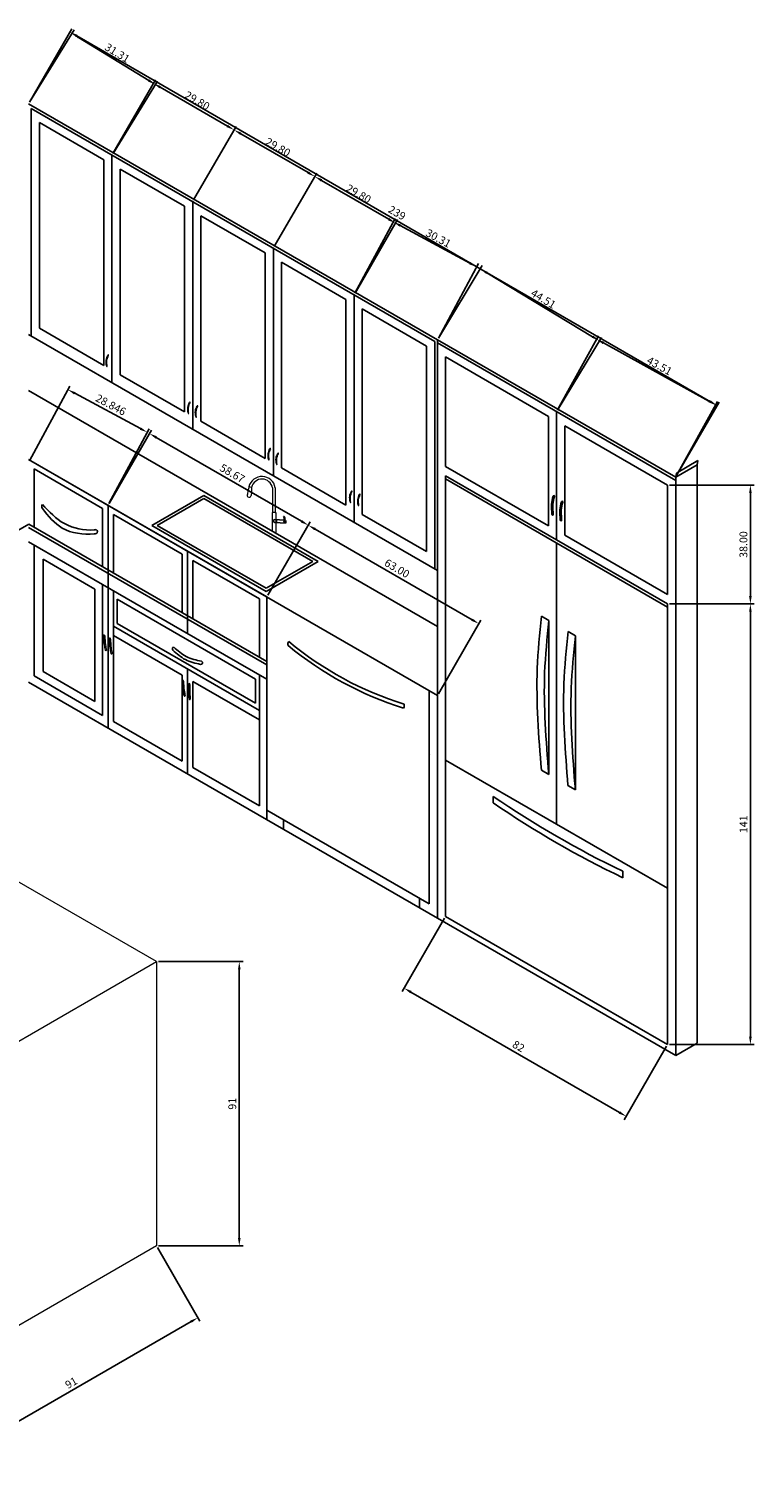
# Model space of a CAD drawing. Units: centimetres. Extents: x 21667 to 22807, y 15845 to 16565.
# Tile 4 of 4: x 22575 to 22807, y 16106 to 16565. Entities that reach past the tile are written whole.
import ezdxf

# ---------------------------------------------------------------- set-up
doc = ezdxf.new("R2010")
doc.units = ezdxf.units.CM
for name, color, linetype, lineweight in [('A-ANNO-DIMS', 2, 'Continuous', 18), ('A-ANNO-NPLT', 8, 'Continuous', 13), ('A-FLOR-FIXT', 4, 'Continuous', 18), ('A-FURN', 8, 'Continuous', 18), ('A-FURN-CASE', 7, 'Continuous', 25), ('A-FURN-HDWR', 8, 'Continuous', 13)]:
    doc.layers.add(name, color=color, linetype=linetype, lineweight=lineweight)
doc.styles.get("Standard").update_dxf_attribs({"font": 'arial.ttf'})
doc.dimstyles.new('ISO-25', dxfattribs={"dimtxt": 2.5, "dimasz": 2.5, "dimexe": 1.25, "dimexo": 0.625, "dimtad": 1, "dimtxsty": 'Standard', "dimcen": 2.5, "dimadec": 0, "dimazin": 0, "dimtfac": 1, "dimtmove": 0, "dimatfit": 3, "dimfxl": 1, "dimarcsym": 0})

# ---------------------------------------------------------------- blocks, each defined once
blk = doc.blocks.new('tabl e3')
for p, q in [((22512.57, 16212.95), (22433.76, 16167.45)), ((22643.34, 16137.45), (22512.57, 16212.95)), ((22433.76, 16167.45), (22564.53, 16091.95)), ((22433.76, 16167.45), (22433.76, 16076.45)), ((22459.07, 16152.84), (22459.07, 16091.06)), ((22564.53, 16091.95), (22643.34, 16137.45)), ((22643.34, 16137.45), (22643.34, 16046.45)), ((22493.36, 16133.04), (22493.36, 16076.26)), ((22495.09, 16132.04), (22495.09, 16075.26)), ((22528.51, 16112.74), (22528.51, 16055.97)), ((22530.25, 16111.74), (22530.25, 16054.97)), ((22459.07, 16096.06), (22564.53, 16035.17)), ((22433.76, 16076.45), (22459.07, 16091.06)), ((22459.07, 16091.06), (22564.53, 16030.17)), ((22564.53, 16000.95), (22564.53, 16091.95)), ((22433.76, 16076.45), (22564.53, 16000.95)), ((22643.34, 16046.45), (22564.53, 16000.95))]:
    blk.add_line(p, q)
for p in [(22494.23, 16132.54), (22529.38, 16112.24)]:
    blk.add_point(p)
blk = doc.blocks.new('PULL-KNOB-A')
for centre, radius, start, end in [((0.27, 0.14), 0.142, 166.0993, 319.2848), ((0.68, 3.52), 0.139, 326.4959, 158.8882)]:
    blk.add_arc(centre, radius, start, end)
for points in [[(0.14, 0.18), (0.04, 0.79), (-0.14, 1.97), (0.33, 3.06), (0.55, 3.57)], [(0.38, 0.05), (0.29, 0.67), (0.11, 1.84), (0.58, 2.93), (0.8, 3.44)]]:
    blk.add_open_spline(points, degree=3, knots=[0, 0, 0, 0, 1.835259, 3.479337, 3.479337, 3.479337, 3.479337])
blk = doc.blocks.new('PULL-KNOB-C')
for centre, radius, start, end in [((0.27, 4.86), 0.21, 340.7069, 183.1566), ((0.41, 0.22), 0.218, 191.5838, 332.2797)]:
    blk.add_arc(centre, radius, start, end)
for points in [[(0.06, 4.85), (0.01, 3.87), (-0.06, 2.31), (0.13, 0.76), (0.2, 0.17)], [(0.46, 4.79), (0.42, 3.82), (0.35, 2.25), (0.54, 0.7), (0.61, 0.12)]]:
    blk.add_open_spline(points, degree=3, knots=[0, 0, 0, 0, 2.913566, 4.680035, 4.680035, 4.680035, 4.680035])
blk = doc.blocks.new('FAUCET')
for p, q in [((1.4, 14.57), (0.59, 14.75)), ((8.15, 14.4), (8.15, 6.62)), ((8.99, 14.47), (8.99, 6.62)), ((8.15, 6.62), (8.01, 6.3)), ((8.01, 6.3), (8.01, 0.66)), ((8.15, 6.62), (8.99, 6.62)), ((8.99, 6.62), (9.15, 6.35)), ((9.15, 6.35), (9.15, 0))]:
    blk.add_line(p, q)
for radius, start in [(4.28, 8.9589), (3.44, 9.9927)]:
    blk.add_arc((4.76, 13.81), radius, start, 167.251)
for points, knots in [([(0.59, 14.75), (0.5, 14.32), (0.32, 13.44), (0.11, 12.57), (0, 12.12)], [0, 0, 0, 0, 1.316127, 2.691834, 2.691834, 2.691834, 2.691834]), ([(1.4, 14.57), (1.41, 14.09), (1.41, 13.24), (1.35, 12.4), (1.32, 12.02)], [0, 0, 0, 0, 1.416831, 2.547877, 2.547877, 2.547877, 2.547877]), ([(0, 12.12), (0.01, 11.98), (0.03, 11.46), (1.13, 11.35), (1.28, 11.86), (1.32, 12.02)], [0, 0, 0, 0, 0.416688, 1.456431, 1.924702, 1.924702, 1.924702, 1.924702])]:
    blk.add_open_spline(points, degree=3, knots=knots)
blk = doc.blocks.new('*D27')
at = {"layer": 'A-ANNO-DIMS', "color": 0, "lineweight": -2, "transparency": 16777216}
for p, q in [((22575.26, 16541.62), (22588.83, 16565.11)), ((22590.37, 16562.77), (22793.02, 16445.77)), ((22782.24, 16422.12), (22795.81, 16445.61))]:
    blk.add_line(p, q, dxfattribs=at)
at = {"layer": 'A-ANNO-DIMS', "color": 0, "transparency": 16777216}
for points in [[(22590.58, 16563.14), (22590.16, 16562.41), (22588.2, 16564.02)], [(22793.23, 16446.14), (22792.81, 16445.41), (22795.18, 16444.52)]]:
    blk.add_solid(points, dxfattribs=at)
at = {"layer": 'Defpoints', "color": 0, "transparency": 16777216}
for p in [(22574.95, 16541.07), (22795.18, 16444.52), (22781.93, 16421.57)]:
    blk.add_point(p, dxfattribs=at)
at = {"layer": 'A-ANNO-DIMS', "color": 0, "transparency": 16777216, "insert": (22692.64, 16505.92), "char_height": 2.5, "attachment_point": 5, "rotation": 330}
blk.add_mtext('239', dxfattribs=at)
blk = doc.blocks.new('*D32')
at = {"layer": 'A-ANNO-DIMS', "color": 0, "lineweight": -2, "transparency": 16777216}
for p, q in [((22708.01, 16280.53), (22694.44, 16257.04)), ((22763.92, 16218.38), (22697.23, 16256.88)), ((22779.02, 16239.53), (22765.46, 16216.04))]:
    blk.add_line(p, q, dxfattribs=at)
at = {"layer": 'A-ANNO-DIMS', "color": 0, "transparency": 16777216}
for points in [[(22697.44, 16257.24), (22697.03, 16256.51), (22695.07, 16258.13)], [(22764.13, 16218.74), (22763.71, 16218.01), (22766.08, 16217.13)]]:
    blk.add_solid(points, dxfattribs=at)
at = {"layer": 'Defpoints', "color": 0, "transparency": 16777216}
for p in [(22708.32, 16281.07), (22695.07, 16258.13), (22779.33, 16240.07)]:
    blk.add_point(p, dxfattribs=at)
at = {"layer": 'A-ANNO-DIMS', "color": 0, "transparency": 16777216, "insert": (22731.53, 16239.27), "char_height": 2.5, "attachment_point": 5, "rotation": 330}
blk.add_mtext('82', dxfattribs=at)
blk = doc.blocks.new('*D33')
at = {"layer": 'A-ANNO-DIMS', "color": 0, "lineweight": -2, "transparency": 16777216}
for p, q in [((22779.96, 16381.07), (22807.08, 16381.07)), ((22805.83, 16378.57), (22805.83, 16242.57)), ((22779.96, 16240.07), (22807.08, 16240.07))]:
    blk.add_line(p, q, dxfattribs=at)
at = {"layer": 'A-ANNO-DIMS', "color": 0, "transparency": 16777216}
for points in [[(22805.42, 16378.57), (22806.25, 16378.57), (22805.83, 16381.07)], [(22805.42, 16242.57), (22806.25, 16242.57), (22805.83, 16240.07)]]:
    blk.add_solid(points, dxfattribs=at)
at = {"layer": 'Defpoints', "color": 0, "transparency": 16777216}
for p in [(22779.33, 16381.07), (22779.33, 16240.07), (22805.83, 16240.07)]:
    blk.add_point(p, dxfattribs=at)
at = {"layer": 'A-ANNO-DIMS', "color": 0, "transparency": 16777216, "insert": (22803.95, 16310.57), "char_height": 2.5, "attachment_point": 5, "rotation": 90}
blk.add_mtext('141', dxfattribs=at)
blk = doc.blocks.new('*D35')
at = {"layer": 'A-ANNO-DIMS', "color": 0, "lineweight": -2, "transparency": 16777216}
for p, q in [((22616.15, 16175.11), (22629.72, 16151.62)), ((22626.93, 16151.45), (22552.45, 16108.45)), ((22537.35, 16129.61), (22550.91, 16106.12))]:
    blk.add_line(p, q, dxfattribs=at)
at = {"layer": 'A-ANNO-DIMS', "color": 0, "transparency": 16777216}
for points in [[(22626.72, 16151.81), (22627.14, 16151.09), (22629.09, 16152.7)], [(22552.24, 16108.81), (22552.66, 16108.09), (22550.28, 16107.2)]]:
    blk.add_solid(points, dxfattribs=at)
at = {"layer": 'Defpoints', "color": 0, "transparency": 16777216}
for p in [(22615.84, 16175.65), (22537.03, 16130.15), (22550.28, 16107.2)]:
    blk.add_point(p, dxfattribs=at)
at = {"layer": 'A-ANNO-DIMS', "color": 0, "transparency": 16777216, "insert": (22588.74, 16131.59), "char_height": 2.5, "attachment_point": 5, "rotation": 30}
blk.add_mtext('91', dxfattribs=at)
blk = doc.blocks.new('*D36')
at = {"layer": 'A-ANNO-DIMS', "color": 0, "lineweight": -2, "transparency": 16777216}
for p, q in [((22616.47, 16266.65), (22643.59, 16266.65)), ((22642.34, 16264.15), (22642.34, 16178.15)), ((22616.47, 16175.65), (22643.59, 16175.65))]:
    blk.add_line(p, q, dxfattribs=at)
at = {"layer": 'A-ANNO-DIMS', "color": 0, "transparency": 16777216}
for points in [[(22641.93, 16264.15), (22642.76, 16264.15), (22642.34, 16266.65)], [(22641.93, 16178.15), (22642.76, 16178.15), (22642.34, 16175.65)]]:
    blk.add_solid(points, dxfattribs=at)
at = {"layer": 'Defpoints', "color": 0, "transparency": 16777216}
for p in [(22615.84, 16266.65), (22615.84, 16175.65), (22642.34, 16175.65)]:
    blk.add_point(p, dxfattribs=at)
at = {"layer": 'A-ANNO-DIMS', "color": 0, "transparency": 16777216, "insert": (22640.44, 16221.15), "char_height": 2.5, "attachment_point": 5, "rotation": 90}
blk.add_mtext('91', dxfattribs=at)
blk = doc.blocks.new('*D62')
at = {"layer": 'A-ANNO-DIMS', "color": 0, "lineweight": -2, "transparency": 16777216}
for p, q in [((22575.28, 16541.61), (22589.49, 16564.71)), ((22590.96, 16562.34), (22613.38, 16548.56)), ((22601.95, 16525.21), (22616.16, 16548.31))]:
    blk.add_line(p, q, dxfattribs=at)
at = {"layer": 'A-ANNO-DIMS', "color": 0, "transparency": 16777216}
for points in [[(22591.18, 16562.69), (22590.74, 16561.99), (22588.83, 16563.65)], [(22613.59, 16548.91), (22613.16, 16548.2), (22615.51, 16547.25)]]:
    blk.add_solid(points, dxfattribs=at)
at = {"layer": 'Defpoints', "color": 0, "transparency": 16777216}
for p in [(22615.51, 16547.25), (22574.95, 16541.07), (22601.63, 16524.67)]:
    blk.add_point(p, dxfattribs=at)
at = {"layer": 'A-ANNO-DIMS', "color": 0, "transparency": 16777216, "insert": (22603.16, 16557.07), "char_height": 2.5, "attachment_point": 5, "rotation": 328.4151}
blk.add_mtext('31.31', dxfattribs=at)
blk = doc.blocks.new('*D63')
at = {"layer": 'A-ANNO-DIMS', "color": 0, "lineweight": -2, "transparency": 16777216}
for p, q in [((22601.94, 16525.22), (22615.5, 16548.71)), ((22617.04, 16546.37), (22638.52, 16533.97)), ((22627.75, 16510.32), (22641.31, 16533.81))]:
    blk.add_line(p, q, dxfattribs=at)
at = {"layer": 'A-ANNO-DIMS', "color": 0, "transparency": 16777216}
for points in [[(22617.25, 16546.74), (22616.83, 16546.01), (22614.88, 16547.62)], [(22638.73, 16534.34), (22638.31, 16533.61), (22640.68, 16532.72)]]:
    blk.add_solid(points, dxfattribs=at)
at = {"layer": 'Defpoints', "color": 0, "transparency": 16777216}
for p in [(22640.68, 16532.72), (22601.63, 16524.67), (22627.43, 16509.77)]:
    blk.add_point(p, dxfattribs=at)
at = {"layer": 'A-ANNO-DIMS', "color": 0, "transparency": 16777216, "insert": (22628.73, 16541.82), "char_height": 2.5, "attachment_point": 5, "rotation": 330}
blk.add_mtext('29.80', dxfattribs=at)
blk = doc.blocks.new('*D64')
at = {"layer": 'A-ANNO-DIMS', "color": 0, "lineweight": -2, "transparency": 16777216}
for p, q in [((22627.75, 16510.32), (22641.31, 16533.81)), ((22642.85, 16531.47), (22664.33, 16519.07)), ((22653.55, 16495.42), (22667.12, 16518.91))]:
    blk.add_line(p, q, dxfattribs=at)
at = {"layer": 'A-ANNO-DIMS', "color": 0, "transparency": 16777216}
for points in [[(22643.06, 16531.84), (22642.64, 16531.11), (22640.68, 16532.72)], [(22664.53, 16519.44), (22664.12, 16518.71), (22666.49, 16517.82)]]:
    blk.add_solid(points, dxfattribs=at)
at = {"layer": 'Defpoints', "color": 0, "transparency": 16777216}
for p in [(22666.49, 16517.82), (22627.43, 16509.77), (22653.24, 16494.87)]:
    blk.add_point(p, dxfattribs=at)
at = {"layer": 'A-ANNO-DIMS', "color": 0, "transparency": 16777216, "insert": (22654.54, 16526.92), "char_height": 2.5, "attachment_point": 5, "rotation": 330}
blk.add_mtext('29.80', dxfattribs=at)
blk = doc.blocks.new('*D65')
at = {"layer": 'A-ANNO-DIMS', "color": 0, "lineweight": -2, "transparency": 16777216}
for p, q in [((22653.55, 16495.42), (22667.12, 16518.91)), ((22668.66, 16516.57), (22690.13, 16504.17)), ((22679.36, 16480.52), (22692.92, 16504.01))]:
    blk.add_line(p, q, dxfattribs=at)
at = {"layer": 'A-ANNO-DIMS', "color": 0, "transparency": 16777216}
for points in [[(22668.86, 16516.94), (22668.45, 16516.21), (22666.49, 16517.82)], [(22690.34, 16504.54), (22689.92, 16503.81), (22692.3, 16502.92)]]:
    blk.add_solid(points, dxfattribs=at)
at = {"layer": 'Defpoints', "color": 0, "transparency": 16777216}
for p in [(22692.3, 16502.92), (22653.24, 16494.87), (22679.05, 16479.97)]:
    blk.add_point(p, dxfattribs=at)
at = {"layer": 'A-ANNO-DIMS', "color": 0, "transparency": 16777216, "insert": (22680.35, 16512.02), "char_height": 2.5, "attachment_point": 5, "rotation": 330}
blk.add_mtext('29.80', dxfattribs=at)
blk = doc.blocks.new('*D66')
at = {"layer": 'A-ANNO-DIMS', "color": 0, "lineweight": -2, "transparency": 16777216}
for p, q in [((22679.35, 16480.52), (22692.23, 16504.39)), ((22693.84, 16502.11), (22716.11, 16490.08)), ((22706.02, 16466.12), (22718.9, 16489.99))]:
    blk.add_line(p, q, dxfattribs=at)
at = {"layer": 'A-ANNO-DIMS', "color": 0, "transparency": 16777216}
for points in [[(22694.03, 16502.47), (22693.64, 16501.74), (22691.64, 16503.29)], [(22716.31, 16490.45), (22715.91, 16489.71), (22718.31, 16488.89)]]:
    blk.add_solid(points, dxfattribs=at)
at = {"layer": 'Defpoints', "color": 0, "transparency": 16777216}
for p in [(22718.31, 16488.89), (22679.05, 16479.97), (22705.72, 16465.57)]:
    blk.add_point(p, dxfattribs=at)
at = {"layer": 'A-ANNO-DIMS', "color": 0, "transparency": 16777216, "insert": (22705.88, 16497.77), "char_height": 2.5, "attachment_point": 5, "rotation": 331.6372}
blk.add_mtext('30.31', dxfattribs=at)
blk = doc.blocks.new('*D67')
at = {"layer": 'A-ANNO-DIMS', "color": 0, "lineweight": -2, "transparency": 16777216}
for p, q in [((22706.04, 16466.11), (22720.06, 16489.33)), ((22721.56, 16486.97), (22755.38, 16466.55)), ((22744.15, 16443.11), (22758.17, 16466.33))]:
    blk.add_line(p, q, dxfattribs=at)
at = {"layer": 'A-ANNO-DIMS', "color": 0, "transparency": 16777216}
for points in [[(22721.77, 16487.33), (22721.34, 16486.61), (22719.42, 16488.26)], [(22755.6, 16466.91), (22755.17, 16466.2), (22757.52, 16465.26)]]:
    blk.add_solid(points, dxfattribs=at)
at = {"layer": 'Defpoints', "color": 0, "transparency": 16777216}
for p in [(22705.72, 16465.57), (22757.52, 16465.26), (22743.83, 16442.57)]:
    blk.add_point(p, dxfattribs=at)
at = {"layer": 'A-ANNO-DIMS', "color": 0, "transparency": 16777216, "insert": (22739.45, 16478.39), "char_height": 2.5, "attachment_point": 5, "rotation": 328.8851}
blk.add_mtext('44.51', dxfattribs=at)
blk = doc.blocks.new('*D68')
at = {"layer": 'A-ANNO-DIMS', "color": 0, "lineweight": -2, "transparency": 16777216}
for p, q in [((22744.13, 16443.12), (22757.22, 16466.88)), ((22758.81, 16464.58), (22792.53, 16445.99)), ((22782.23, 16422.12), (22795.33, 16445.88))]:
    blk.add_line(p, q, dxfattribs=at)
at = {"layer": 'A-ANNO-DIMS', "color": 0, "transparency": 16777216}
for points in [[(22759.01, 16464.94), (22758.61, 16464.21), (22756.62, 16465.78)], [(22792.73, 16446.36), (22792.33, 16445.63), (22794.72, 16444.78)]]:
    blk.add_solid(points, dxfattribs=at)
at = {"layer": 'Defpoints', "color": 0, "transparency": 16777216}
for p in [(22743.83, 16442.57), (22794.72, 16444.78), (22781.93, 16421.57)]:
    blk.add_point(p, dxfattribs=at)
at = {"layer": 'A-ANNO-DIMS', "color": 0, "transparency": 16777216, "insert": (22776.59, 16456.95), "char_height": 2.5, "attachment_point": 5, "rotation": 331.1405}
blk.add_mtext('43.51', dxfattribs=at)
blk = doc.blocks.new('*D75')
at = {"layer": 'A-ANNO-DIMS', "color": 0, "lineweight": -2, "transparency": 16777216}
for p, q in [((22575.25, 16426.85), (22588.1, 16450.74)), ((22589.71, 16448.45), (22610.71, 16437.16)), ((22600.65, 16413.19), (22613.5, 16437.07))]:
    blk.add_line(p, q, dxfattribs=at)
at = {"layer": 'A-ANNO-DIMS', "color": 0, "transparency": 16777216}
for points in [[(22589.91, 16448.82), (22589.51, 16448.09), (22587.51, 16449.64)], [(22610.91, 16437.52), (22610.51, 16436.79), (22612.91, 16435.97)]]:
    blk.add_solid(points, dxfattribs=at)
at = {"layer": 'Defpoints', "color": 0, "transparency": 16777216}
for p in [(22612.91, 16435.97), (22574.95, 16426.3), (22600.36, 16412.64)]:
    blk.add_point(p, dxfattribs=at)
at = {"layer": 'A-ANNO-DIMS', "color": 0, "transparency": 16777216, "insert": (22601.11, 16444.48), "char_height": 2.5, "attachment_point": 5, "rotation": 331.7204}
blk.add_mtext('28.846', dxfattribs=at)
blk = doc.blocks.new('*D76')
at = {"layer": 'A-ANNO-DIMS', "color": 0, "lineweight": -2, "transparency": 16777216}
for p, q in [((22600.67, 16413.18), (22614.23, 16436.67)), ((22615.77, 16434.33), (22662.25, 16407.5)), ((22651.47, 16383.84), (22665.04, 16407.33))]:
    blk.add_line(p, q, dxfattribs=at)
at = {"layer": 'A-ANNO-DIMS', "color": 0, "transparency": 16777216}
for points in [[(22615.98, 16434.7), (22615.56, 16433.97), (22613.61, 16435.58)], [(22662.46, 16407.86), (22662.04, 16407.14), (22664.41, 16406.25)]]:
    blk.add_solid(points, dxfattribs=at)
at = {"layer": 'Defpoints', "color": 0, "transparency": 16777216}
for p in [(22600.36, 16412.64), (22664.41, 16406.25), (22651.16, 16383.3)]:
    blk.add_point(p, dxfattribs=at)
at = {"layer": 'A-ANNO-DIMS', "color": 0, "transparency": 16777216, "insert": (22639.96, 16422.56), "char_height": 2.5, "attachment_point": 5, "rotation": 330}
blk.add_mtext('58.67', dxfattribs=at)
blk = doc.blocks.new('*D77')
at = {"layer": 'A-ANNO-DIMS', "color": 0, "lineweight": -2, "transparency": 16777216}
for p, q in [((22651.47, 16383.84), (22665.04, 16407.33)), ((22666.58, 16405), (22716.81, 16376)), ((22706.03, 16352.34), (22719.6, 16375.83))]:
    blk.add_line(p, q, dxfattribs=at)
at = {"layer": 'A-ANNO-DIMS', "color": 0, "transparency": 16777216}
for points in [[(22666.79, 16405.36), (22666.37, 16404.64), (22664.41, 16406.25)], [(22717.02, 16376.36), (22716.6, 16375.64), (22718.97, 16374.75)]]:
    blk.add_solid(points, dxfattribs=at)
at = {"layer": 'Defpoints', "color": 0, "transparency": 16777216}
for p in [(22651.16, 16383.3), (22718.97, 16374.75), (22705.72, 16351.8)]:
    blk.add_point(p, dxfattribs=at)
at = {"layer": 'A-ANNO-DIMS', "color": 0, "transparency": 16777216, "insert": (22692.64, 16392.15), "char_height": 2.5, "attachment_point": 5, "rotation": 330}
blk.add_mtext('63.00', dxfattribs=at)
blk = doc.blocks.new('*D78')
at = {"layer": 'A-ANNO-DIMS', "color": 0, "lineweight": -2, "transparency": 16777216}
for p, q in [((22779.96, 16419.07), (22807.08, 16419.07)), ((22805.83, 16416.57), (22805.83, 16383.57)), ((22779.96, 16381.07), (22807.08, 16381.07))]:
    blk.add_line(p, q, dxfattribs=at)
at = {"layer": 'A-ANNO-DIMS', "color": 0, "transparency": 16777216}
for points in [[(22805.42, 16416.57), (22806.25, 16416.57), (22805.83, 16419.07)], [(22805.42, 16383.57), (22806.25, 16383.57), (22805.83, 16381.07)]]:
    blk.add_solid(points, dxfattribs=at)
at = {"layer": 'Defpoints', "color": 0, "transparency": 16777216}
for p in [(22779.33, 16419.07), (22779.33, 16381.07), (22805.83, 16381.07)]:
    blk.add_point(p, dxfattribs=at)
at = {"layer": 'A-ANNO-DIMS', "color": 0, "transparency": 16777216, "insert": (22803.93, 16400.07), "char_height": 2.5, "attachment_point": 5, "rotation": 90}
blk.add_mtext('38.00', dxfattribs=at)

msp = doc.modelspace()

# ---------------------------------------------------------------- linework, layer by layer
at = {"layer": 'A-ANNO-NPLT'}
for p in [(22601.6255, 16524.675), (22627.4331, 16509.775), (22653.2406, 16494.875), (22679.0482, 16479.975), (22600.3554, 16412.635), (22625.7588, 16397.9684)]:
    msp.add_point(p, dxfattribs=at)
at = {"layer": 'A-FURN-CASE'}
for p, q in [((22574.9519, 16541.075), (22705.7218, 16465.575)), ((22575.818, 16539.575), (22704.8558, 16465.075)), ((22575.818, 16466.8017), (22575.818, 16539.575)), ((22578.416, 16535.075), (22599.0274, 16523.175)), ((22578.416, 16469.3017), (22578.416, 16535.075)), ((22601.6255, 16524.675), (22601.6255, 16451.9017)), ((22599.0274, 16523.175), (22599.0274, 16457.4017)), ((22604.2236, 16520.175), (22604.2236, 16454.4017)), ((22604.2236, 16520.175), (22624.835, 16508.275)), ((22624.835, 16508.275), (22624.835, 16442.5017)), ((22627.4331, 16509.775), (22627.4331, 16437.0017)), ((22630.0312, 16505.275), (22630.0312, 16439.5017)), ((22630.0312, 16505.275), (22650.6426, 16493.375)), ((22650.6426, 16493.375), (22650.6426, 16427.6017)), ((22653.2406, 16494.875), (22653.2406, 16422.1017)), ((22655.8387, 16490.375), (22655.8387, 16424.6017)), ((22655.8387, 16490.375), (22676.4501, 16478.475)), ((22676.4501, 16478.475), (22676.4501, 16412.7017)), ((22679.0482, 16479.975), (22679.0482, 16407.2017)), ((22681.6463, 16475.475), (22681.6463, 16409.7017)), ((22681.6463, 16475.475), (22702.2577, 16463.575)), ((22578.416, 16469.3017), (22599.0274, 16457.4017)), ((22574.9519, 16467.3017), (22705.7218, 16391.8017)), ((22704.8558, 16465.075), (22704.8558, 16392.3017)), ((22705.7218, 16465.575), (22705.7218, 16391.8017)), ((22705.7218, 16465.575), (22781.932, 16421.575)), ((22705.7218, 16280.575), (22705.7218, 16465.575)), ((22705.7218, 16464.575), (22781.932, 16420.575)), ((22702.2577, 16463.575), (22702.2577, 16397.8017)), ((22708.3199, 16460.075), (22741.2288, 16441.075)), ((22708.3199, 16425.075), (22708.3199, 16460.075)), ((22604.2236, 16454.4017), (22624.835, 16442.5017)), ((22574.9519, 16449.3927), (22705.7218, 16373.8927)), ((22743.8269, 16442.575), (22743.8269, 16401.575)), ((22630.0312, 16439.5017), (22650.6426, 16427.6017)), ((22741.2288, 16441.075), (22741.2288, 16406.075)), ((22746.425, 16438.075), (22746.425, 16403.075)), ((22746.425, 16438.075), (22779.3339, 16419.075)), ((22574.9519, 16427.3017), (22705.7218, 16351.8017)), ((22574.9519, 16427.3017), (22651.1622, 16383.3017)), ((22576.684, 16424.3017), (22598.6233, 16411.635)), ((22576.684, 16424.3017), (22576.684, 16405.6387)), ((22655.8387, 16424.6017), (22676.4501, 16412.7017)), ((22708.3199, 16425.075), (22741.2288, 16406.075)), ((22781.932, 16421.575), (22788.8602, 16425.575)), ((22781.932, 16421.575), (22782.1981, 16422.95)), ((22782.1981, 16422.95), (22789.056, 16426.9863)), ((22788.8602, 16425.575), (22789.056, 16426.9863)), ((22788.8602, 16240.575), (22788.8602, 16425.575)), ((22708.3199, 16281.075), (22708.3199, 16422.075)), ((22708.3199, 16422.075), (22779.3339, 16381.075)), ((22708.3199, 16421.075), (22779.3339, 16380.075)), ((22779.3339, 16419.075), (22779.3339, 16384.075)), ((22781.932, 16421.575), (22781.932, 16236.575)), ((22631.0558, 16415.8072), (22614.3716, 16406.1746)), ((22631.0558, 16414.8072), (22616.1037, 16406.1746)), ((22667.6266, 16394.6931), (22631.0558, 16415.8072)), ((22665.8945, 16394.6931), (22631.0558, 16414.8072)), ((22598.6233, 16411.635), (22598.6233, 16392.9721)), ((22600.3554, 16412.635), (22600.3554, 16341.4083)), ((22602.0874, 16409.635), (22602.0874, 16390.9721)), ((22602.0874, 16409.635), (22624.0267, 16396.9684)), ((22681.6463, 16409.7017), (22702.2577, 16397.8017)), ((22403.0888, 16307.3461), (22575.0103, 16406.605)), ((22574.9519, 16405.5595), (22651.1622, 16361.5595)), ((22575.0103, 16406.605), (22651.1622, 16362.6387)), ((22650.9424, 16385.0605), (22614.3716, 16406.1746)), ((22650.9424, 16386.0605), (22616.1037, 16406.1746)), ((22653.506, 16408.12), (22656.9269, 16407.9165)), ((22653.6991, 16407.1344), (22657.1177, 16406.9309)), ((22574.9519, 16400.9426), (22598.6233, 16387.2759)), ((22576.684, 16399.9426), (22576.684, 16358.075)), ((22743.8269, 16400.575), (22743.8269, 16310.575)), ((22746.425, 16403.075), (22779.3339, 16384.075)), ((22579.5751, 16395.3401), (22596.0953, 16385.8022)), ((22579.5751, 16395.3401), (22579.5751, 16359.4058)), ((22624.0267, 16396.9684), (22624.0267, 16378.3054)), ((22625.7588, 16397.9684), (22625.7588, 16371.6092)), ((22627.4908, 16394.9684), (22627.4908, 16376.3054)), ((22627.4908, 16394.9684), (22648.8032, 16382.6637)), ((22650.9424, 16385.0605), (22667.6266, 16394.6931)), ((22650.9424, 16386.0605), (22665.8945, 16394.6931)), ((22598.6233, 16387.2759), (22624.0267, 16372.6092)), ((22598.6233, 16387.2759), (22598.6233, 16345.4083)), ((22596.0953, 16385.8022), (22596.0953, 16349.8678)), ((22602.0874, 16385.2759), (22602.0874, 16343.4083)), ((22603.2287, 16374.8477), (22603.2287, 16382.572)), ((22603.2287, 16382.572), (22647.5238, 16356.9982)), ((22648.8032, 16382.6637), (22648.8032, 16364.0007)), ((22651.1622, 16383.3017), (22651.1622, 16312.075)), ((22739.0034, 16377.1069), (22741.3587, 16375.747)), ((22779.3339, 16381.075), (22779.3339, 16240.075)), ((22648.8032, 16346.9669), (22602.0874, 16373.9383)), ((22647.5238, 16349.2739), (22603.2287, 16374.8477)), ((22624.0267, 16372.6092), (22651.1622, 16356.9426)), ((22741.3587, 16375.747), (22741.3347, 16326.5322)), ((22624.0267, 16358.2717), (22602.0874, 16370.9383)), ((22747.5058, 16372.198), (22749.8611, 16370.8382)), ((22749.8611, 16370.8382), (22749.8371, 16321.6233)), ((22596.0953, 16349.8678), (22579.5751, 16359.4058)), ((22625.7588, 16360.2717), (22625.7588, 16326.7416)), ((22705.7218, 16280.575), (22574.9519, 16356.075)), ((22598.6233, 16345.4083), (22576.684, 16358.075)), ((22624.0267, 16358.2717), (22624.0267, 16330.7416)), ((22627.4908, 16356.2717), (22627.4908, 16328.7416)), ((22648.8032, 16343.9669), (22627.4908, 16356.2717)), ((22647.5238, 16356.9982), (22647.5238, 16349.2739)), ((22648.8032, 16358.3045), (22648.8032, 16316.4369)), ((22703.1237, 16353.3017), (22703.1237, 16285.075)), ((22705.7218, 16351.8017), (22705.7218, 16280.575)), ((22624.0267, 16330.7416), (22602.0874, 16343.4083)), ((22703.1237, 16332.6387), (22703.2832, 16332.5467)), ((22779.3339, 16290.075), (22708.3199, 16331.075)), ((22648.8032, 16316.4369), (22627.4908, 16328.7416)), ((22741.3347, 16326.5322), (22738.9794, 16327.892)), ((22749.8371, 16321.6233), (22747.4818, 16322.9832)), ((22723.5671, 16317.4087), (22723.5671, 16319.5003)), ((22703.1237, 16285.075), (22651.1622, 16315.075)), ((22656.5381, 16311.9712), (22656.5381, 16308.9712)), ((22765.0143, 16293.4791), (22765.0143, 16295.5707)), ((22699.9361, 16286.9153), (22699.9361, 16283.9153)), ((22781.932, 16236.575), (22705.7218, 16280.575)), ((22779.3339, 16240.075), (22708.3199, 16281.075)), ((22781.932, 16236.575), (22788.8602, 16240.575))]:
    msp.add_line(p, q, dxfattribs=at)
for centre, radius, start, end in [((22742.932, 16415.483), 0.2369, 349.827552, 167.607275), ((22745.614, 16413.6633), 0.2369, 349.827552, 167.607275), ((22580.1657, 16412.251), 1.0244, 141.888843, 218.111157), ((22656.6106, 16408.9632), 0.1083, 11.472802, 160.933429), ((22654.3486, 16407.9945), 2.3816, 343.073014, 24.934412), ((22654.5571, 16407.9807), 2.3816, 343.073014, 24.934412), ((22742.5954, 16409.7601), 0.2913, 197.962885, 304.739292), ((22596.333, 16404.1986), 0.6675, 288.710977, 71.289023), ((22653.8655, 16407.6787), 0.5692, 129.168141, 253.001145), ((22653.3327, 16407.51), 0.8739, 332.759171, 41.722153), ((22656.7396, 16407.4198), 0.1636, 226.514294, 305.891937), ((22656.6738, 16407.3562), 0.6148, 316.230119, 65.688838), ((22745.2774, 16407.9404), 0.2913, 197.962885, 304.739292), ((22658.9133, 16368.2502), 1.0504, 133.593574, 208.092042), ((22727.2848, 16451.3997), 108.6213, 230.358642, 252.620983), ((22727.4872, 16452.6551), 108.6213, 230.358642, 252.620983), ((22621.544, 16366.6808), 0.6058, 103.584302, 221.520852), ((22630.0415, 16362.2418), 0.5293, 263.783382, 61.321772), ((22694.004, 16348.5158), 1.143, 317.045708, 24.639907), ((22898.3838, 16574.4326), 309.1138, 235.560089, 244.439911), ((22898.3838, 16572.3409), 309.1138, 235.560089, 244.439911)]:
    msp.add_arc(centre, radius, start, end, dxfattribs=at)
for points, knots in [([(22742.3183, 16409.6703), (22742.2841, 16410.3766), (22742.2305, 16411.4863), (22742.1827, 16413.4724), (22742.4767, 16414.7133), (22742.7069, 16415.5566)], [0, 0, 0, 0, 2.12371012, 3.33605011, 5.93696928, 5.93696928, 5.93696928, 5.93696928]), ([(22742.7622, 16409.5026), (22742.7281, 16410.209), (22742.6745, 16411.3186), (22742.6262, 16413.3226), (22742.929, 16414.5806), (22743.1651, 16415.4412)], [0, 0, 0, 0, 2.12371012, 3.33605011, 5.99070247, 5.99070247, 5.99070247, 5.99070247]), ([(22745.0003, 16407.8505), (22744.9662, 16408.5569), (22744.9125, 16409.6665), (22744.8647, 16411.6526), (22745.1588, 16412.8936), (22745.3889, 16413.7369)], [0, 0, 0, 0, 2.12371012, 3.33605011, 5.93696928, 5.93696928, 5.93696928, 5.93696928]), ([(22745.4443, 16407.6828), (22745.4101, 16408.3892), (22745.3565, 16409.4989), (22745.3082, 16411.5029), (22745.6111, 16412.7609), (22745.8471, 16413.6214)], [0, 0, 0, 0, 2.12371012, 3.33605011, 5.99070247, 5.99070247, 5.99070247, 5.99070247]), ([(22579.3597, 16412.8833), (22581.5195, 16410.5876), (22585.9345, 16405.8947), (22592.9028, 16404.4321), (22596.3352, 16404.8076), (22596.5471, 16404.8308)], [0, 0, 0, 0, 9.31388704, 19.03956177, 19.67959192, 19.67959192, 19.67959192, 19.67959192]), ([(22579.3597, 16411.6188), (22581.2747, 16409.2128), (22585.4001, 16404.0298), (22592.7035, 16403.154), (22596.3353, 16403.5436), (22596.5471, 16403.5664)], [0, 0, 0, 0, 8.95443098, 19.28977515, 19.9298053, 19.9298053, 19.9298053, 19.9298053]), ([(22739.0034, 16377.1069), (22738.4452, 16371.5352), (22736.805, 16355.1623), (22738.1151, 16338.7315), (22738.9794, 16327.892)], [0, 0, 0, 0, 16.77466817, 49.29421568, 49.29421568, 49.29421568, 49.29421568]), ([(22741.3587, 16375.747), (22740.8005, 16370.1754), (22739.1603, 16353.8025), (22740.4704, 16337.3717), (22741.3347, 16326.5322)], [0, 0, 0, 0, 16.77466817, 49.29421568, 49.29421568, 49.29421568, 49.29421568]), ([(22747.5058, 16372.198), (22746.9476, 16366.6264), (22745.3074, 16350.2535), (22746.6175, 16333.8226), (22747.4818, 16322.9832)], [0, 0, 0, 0, 16.77466817, 49.29421568, 49.29421568, 49.29421568, 49.29421568]), ([(22749.8611, 16370.8382), (22749.3029, 16365.2665), (22747.6627, 16348.8936), (22748.9728, 16332.4628), (22749.8371, 16321.6233)], [0, 0, 0, 0, 16.77466817, 49.29421568, 49.29421568, 49.29421568, 49.29421568]), ([(22621.0904, 16366.2792), (22622.358, 16365.1436), (22624.9225, 16362.8464), (22628.2842, 16362.0954), (22629.9842, 16361.7157)], [0, 0, 0, 0, 5.01561683, 10.14656144, 10.14656144, 10.14656144, 10.14656144]), ([(22621.4017, 16367.2697), (22622.6693, 16366.1341), (22625.2338, 16363.8368), (22628.5955, 16363.0859), (22630.2955, 16362.7062)], [0, 0, 0, 0, 5.01561683, 10.14656144, 10.14656144, 10.14656144, 10.14656144])]:
    msp.add_open_spline(points, degree=3, knots=knots, dxfattribs=at)

# ---------------------------------------------------------------- block references
at = {"layer": 'A-FLOR-FIXT'}
msp.add_blockref('FAUCET', (22644.8389, 16403.7627), dxfattribs=at)
at = {"layer": 'A-FURN'}
msp.add_blockref('tabl e3', (-27.5005, 129.1994), dxfattribs=at)
at = {"layer": 'A-FURN-HDWR'}
for name, p in [('PULL-KNOB-A', (22599.733, 16457.065)), ('PULL-KNOB-A', (22625.834, 16441.9956)), ('PULL-KNOB-A', (22628.2752, 16440.8105)), ('PULL-KNOB-A', (22651.5655, 16427.1395)), ('PULL-KNOB-A', (22654.0748, 16425.6908)), ('PULL-KNOB-A', (22677.6388, 16413.5431)), ('PULL-KNOB-A', (22680.2369, 16412.5188)), ('PULL-KNOB-C', (22626.07, 16350.501))]:
    msp.add_blockref(name, p, dxfattribs=at)
for p, rotation in [((22599.2562, 16366.072), 4.614980082148825), ((22601.0633, 16365.0286), 4.614980082145505), ((22624.445, 16351.5292), 4.614980081989283)]:
    msp.add_blockref('PULL-KNOB-C', p, dxfattribs=dict(at, rotation=rotation))

# ---------------------------------------------------------------- dimensions: what is measured, and where the dimension line sits
at = {"layer": 'A-ANNO-DIMS'}
for base, p1, p2, angle, override, picture, middle in [((22795.182, 16444.5246), (22574.9519, 16541.075), (22781.932, 16421.575), 330, {"dimdec": 0, "dimlfac": 1, "dimrnd": 0, "dimzin": 0, "dimdsep": 46, "dimlunit": 2}, '*D27', (22692.6431, 16505.9221)), ((22615.5052, 16547.2494), (22574.9519, 16541.075), (22601.6255, 16524.675), 328.415114, {"dimdec": 2, "dimlfac": 1, "dimrnd": 0, "dimzin": 0, "dimdsep": 46, "dimlunit": 2}, '*D62', (22603.1647, 16557.0699)), ((22640.6831, 16532.7246), (22601.6255, 16524.675), (22627.4331, 16509.775), 330, {"dimdec": 2, "dimlfac": 1, "dimrnd": 0, "dimzin": 0, "dimdsep": 46, "dimlunit": 2}, '*D63', (22628.73, 16541.8213)), ((22666.4906, 16517.8246), (22627.4331, 16509.775), (22653.2406, 16494.875), 330, {"dimdec": 2, "dimlfac": 1, "dimrnd": 0, "dimzin": 0, "dimdsep": 46, "dimlunit": 2}, '*D64', (22654.5376, 16526.9213)), ((22692.2982, 16502.9246), (22653.2406, 16494.875), (22679.0482, 16479.975), 330, {"dimdec": 2, "dimlfac": 1, "dimrnd": 0, "dimzin": 0, "dimdsep": 46, "dimlunit": 2}, '*D65', (22680.3451, 16512.0213)), ((22718.3107, 16488.8938), (22679.0482, 16479.975), (22705.7218, 16465.575), 331.637165, {"dimdec": 2, "dimlfac": 1, "dimrnd": 0, "dimzin": 0, "dimdsep": 46, "dimlunit": 2}, '*D66', (22705.8776, 16497.7677)), ((22757.5209, 16465.2625), (22705.7218, 16465.575), (22743.8269, 16442.575), 328.885094, {"dimdec": 2, "dimlfac": 1, "dimrnd": 0, "dimzin": 0, "dimdsep": 46, "dimlunit": 2}, '*D67', (22739.4509, 16478.3904)), ((22794.7226, 16444.7838), (22743.8269, 16442.575), (22781.932, 16421.575), 331.14053, {"dimdec": 2, "dimlfac": 1, "dimrnd": 0, "dimzin": 0, "dimdsep": 46, "dimlunit": 2}, '*D68', (22776.5882, 16456.9499)), ((22612.9104, 16435.9722), (22574.9519, 16426.3017), (22600.3554, 16412.635), 331.720394, {"dimdec": 3, "dimlfac": 1, "dimrnd": 0, "dimzin": 0, "dimdsep": 46, "dimlunit": 2}, '*D75', (22601.1095, 16444.48)), ((22664.4122, 16406.2514), (22600.3554, 16412.635), (22651.1622, 16383.3017), 330, {"dimdec": 2, "dimlfac": 1, "dimrnd": 0, "dimzin": 0, "dimdsep": 46, "dimlunit": 2}, '*D76', (22639.9595, 16422.5647)), ((22805.8339, 16381.075), (22779.3339, 16419.075), (22779.3339, 16381.075), 270, {"dimdec": 2, "dimlfac": 1, "dimrnd": 0, "dimzin": 0, "dimdsep": 46, "dimlunit": 2}, '*D78', (22803.9317, 16400.075)), ((22718.9718, 16374.7514), (22651.1622, 16383.3017), (22705.7218, 16351.8017), 330, {"dimdec": 2, "dimlfac": 1, "dimrnd": 0, "dimzin": 0, "dimdsep": 46, "dimlunit": 2}, '*D77', (22692.6431, 16392.1488)), ((22805.8339, 16240.075), (22779.3339, 16381.075), (22779.3339, 16240.075), 270, {"dimdec": 0, "dimlfac": 1, "dimrnd": 0, "dimzin": 0, "dimdsep": 46, "dimlunit": 2}, '*D33', (22803.9538, 16310.575)), ((22695.0699, 16258.1253), (22779.3339, 16240.075), (22708.3199, 16281.075), 150, {"dimdec": 0, "dimlfac": 1, "dimrnd": 0, "dimzin": 0, "dimdsep": 46, "dimlunit": 2}, '*D32', (22731.5276, 16239.272)), ((22642.3418, 16175.6477), (22615.8418, 16266.6477), (22615.8418, 16175.6477), 270, {"dimdec": 0, "dimlfac": 1, "dimrnd": 0, "dimzin": 0, "dimdsep": 46, "dimlunit": 2}, '*D36', (22640.4404, 16221.1477)), ((22550.2835, 16107.198), (22615.8418, 16175.6477), (22537.0335, 16130.1477), 210, {"dimdec": 0, "dimlfac": 1, "dimrnd": 0, "dimzin": 0, "dimdsep": 46, "dimlunit": 2}, '*D35', (22588.737, 16131.5947))]:
    dim = msp.add_linear_dim(base=base, p1=p1, p2=p2, angle=angle, dimstyle='ISO-25', override=override, dxfattribs=at)
    dim.commit()
    dim.dimension.update_dxf_attribs({"geometry": picture, "text_midpoint": middle})

doc.saveas('drawing.dxf')
